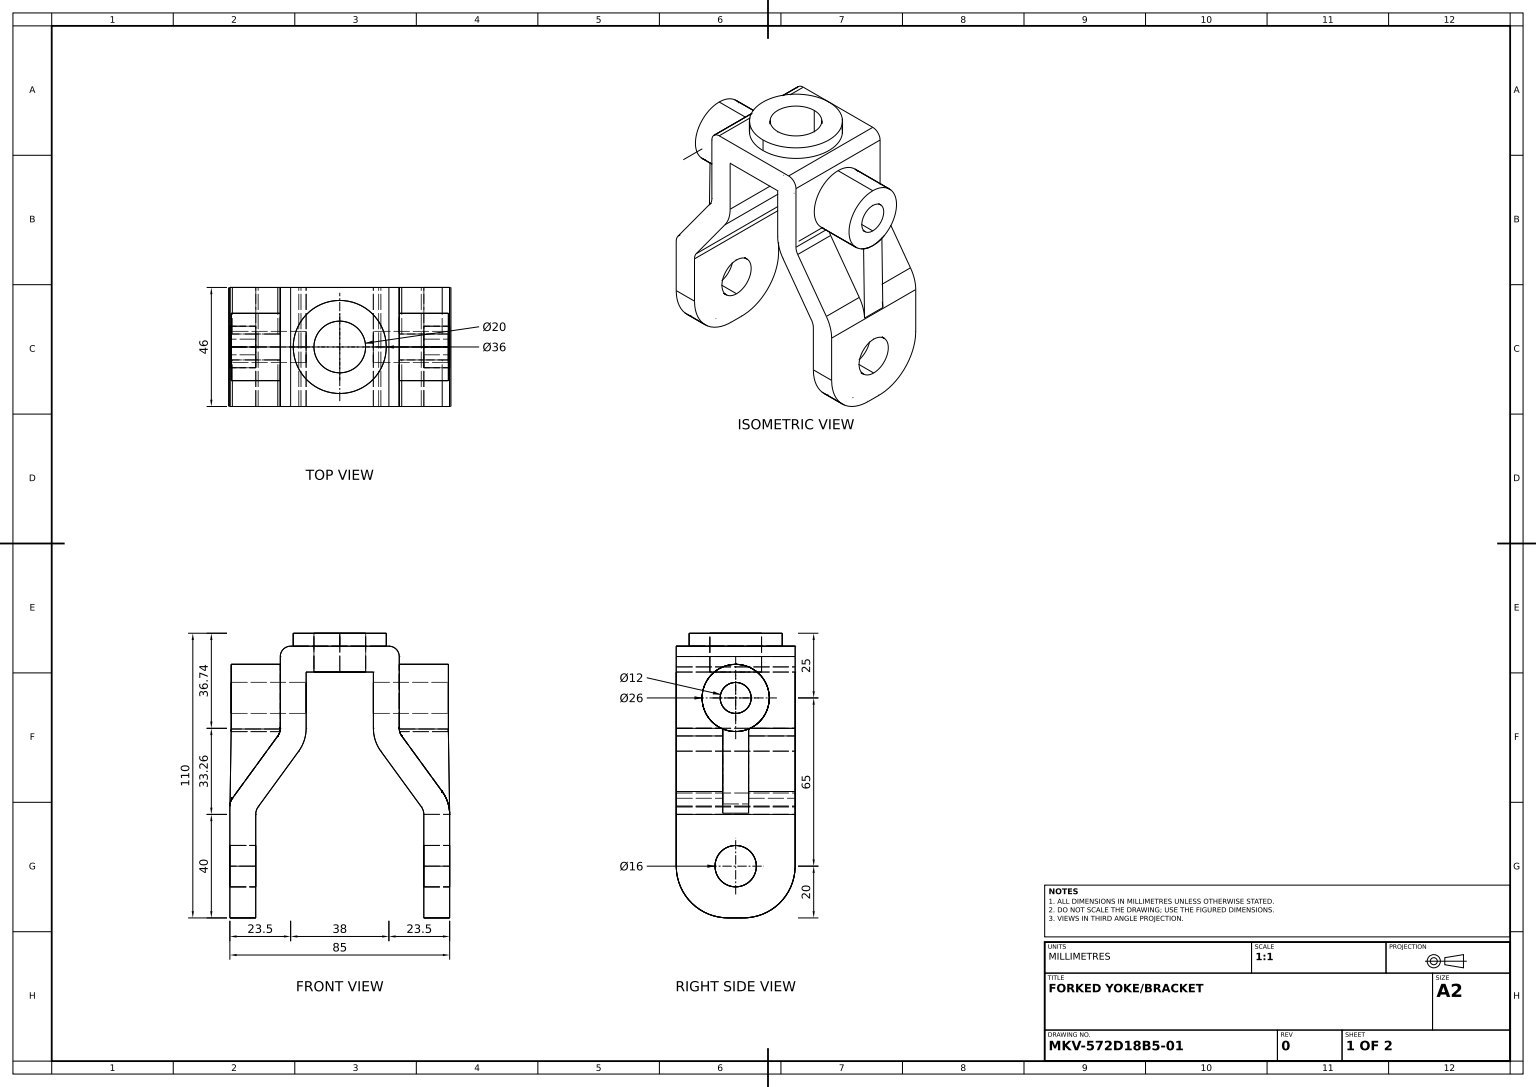
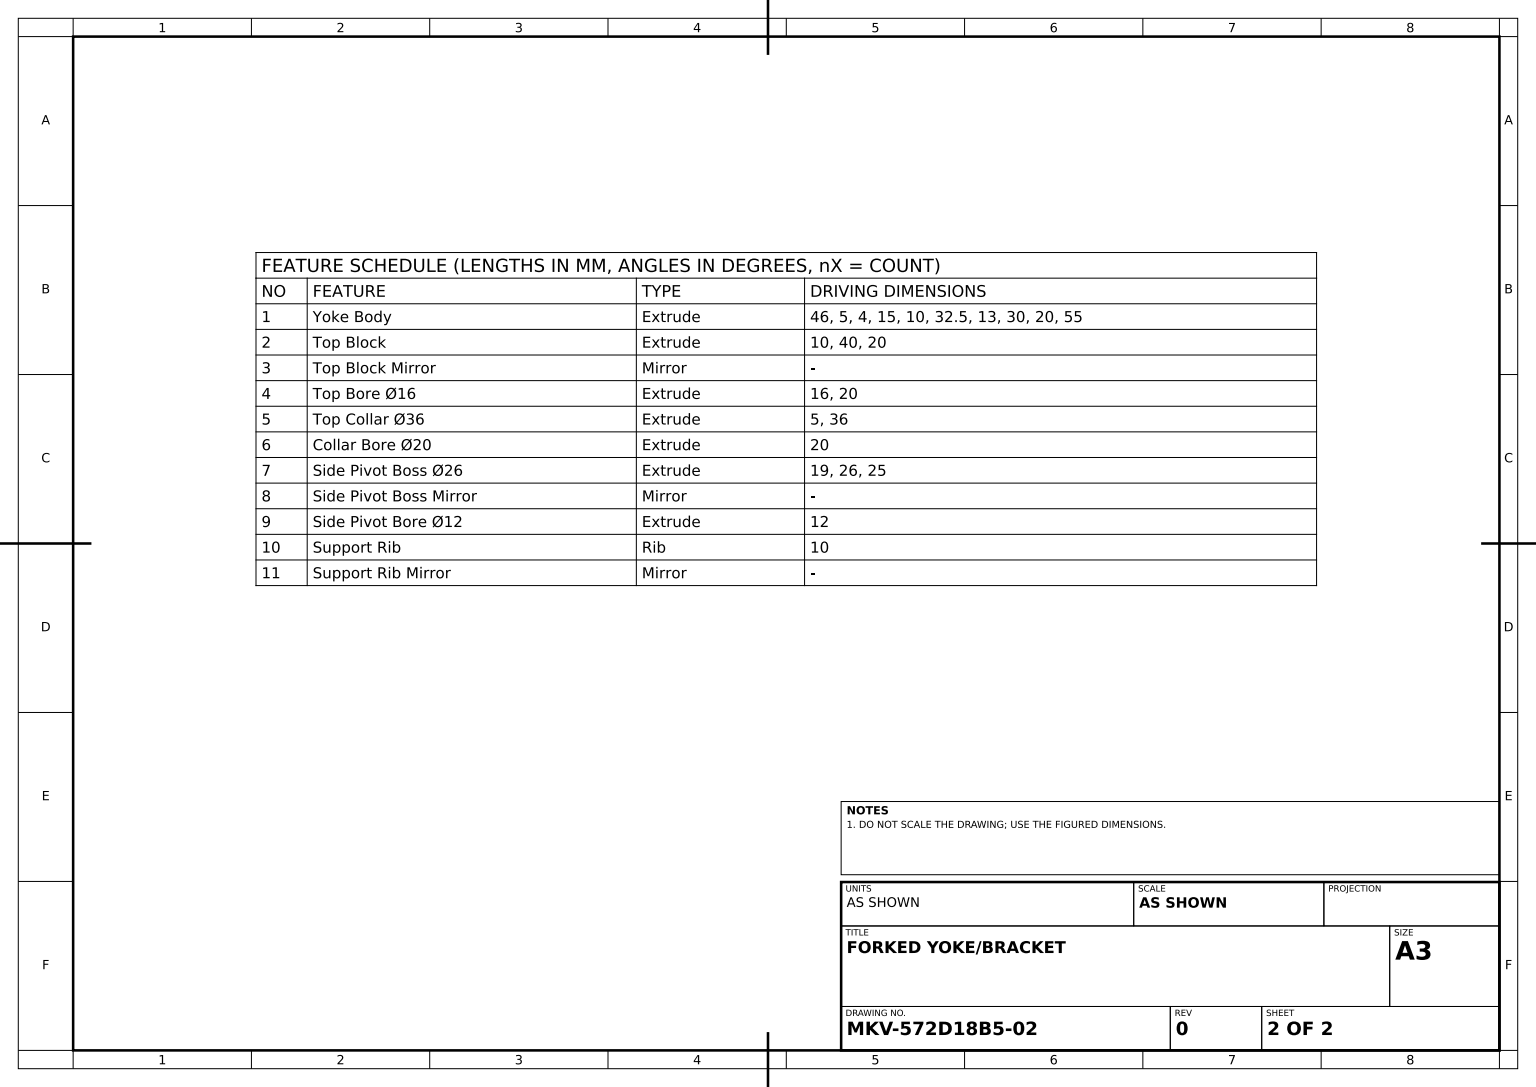
from build123d import *

# Parameters (mm, degrees)
YOKE_BODY_DEPTH           = 23
TOP_BLOCK_DEPTH           = 10
TOP_BORE_SKETCH_R         = 8
TOP_BORE_16_DEPTH         = 130.533779378
TOP_COLLAR_SKETCH_R       = 18
TOP_COLLAR_36_DEPTH       = 5
COLLAR_BORE_20_REACH      = 122.147
COLLAR_BORE_SKETCH_R      = 10
SIDE_PIVOT_BOSS_SKETCH_R  = 13
SIDE_PIVOT_BOSS_26_DEPTH  = 19
SIDE_PIVOT_BORE_SKETCH_R  = 6
SIDE_PIVOT_BORE_12_DEPTH  = 130.206230518
SUPPORT_RIB_REACH         = 108.584
SUPPORT_RIB_SKETCH_WALL_W = 247.172853136
SUPPORT_RIB_SKETCH_WALL_H = 10


with BuildPart() as part:
    # Yoke Profile Sketch → Yoke Body (new, symmetric)
    with BuildSketch(Plane.XY):
        with BuildLine():
            Line((19, 10), (-19, 10))
            ThreePointArc((-19, 10), (-21.828427125, 8.828427125), (-23, 6))
            Line((-23, 6), (-23, -21.741149913))
            ThreePointArc((-23, -21.741149913), (-23.246067912, -23.290385113), (-23.960051881, -24.687133484))
            Line((-23.960051881, -24.687133484), (-41.539948119, -48.795166343))
            ThreePointArc((-41.539948119, -48.795166343), (-42.253932088, -50.191914714), (-42.5, -51.741149913))
            Line((-42.5, -51.741149913), (-42.5, -71.741149913))
            Line((-42.5, -71.741149913), (-32.5, -71.741149913))
            Line((-32.5, -71.741149913), (-32.5, -55))
            ThreePointArc((-32.5, -55), (-32.253932088, -53.4507648), (-31.539948119, -52.054016429))
            Line((-31.539948119, -52.054016429), (-15.880155644, -30.579100626))
            ThreePointArc((-15.880155644, -30.579100626), (-13.738203736, -26.388855512), (-13, -21.741149913))
            Line((-13, -21.741149913), (-13, 0))
            Line((-13, 0), (13, 0))
            Line((13, 0), (13, -21.741149913))
            ThreePointArc((13, -21.741149913), (13.738203736, -26.388855512), (15.880155644, -30.579100626))
            Line((15.880155644, -30.579100626), (31.539948119, -52.054016429))
            ThreePointArc((31.539948119, -52.054016429), (32.253932088, -53.4507648), (32.5, -55))
            Line((32.5, -55), (32.5, -71.741149913))
            Line((32.5, -71.741149913), (42.5, -71.741149913))
            Line((42.5, -71.741149913), (42.5, -55))
            ThreePointArc((42.5, -55), (41.761796264, -50.352294401), (39.619844356, -46.162049287))
            Line((39.619844356, -46.162049287), (23.960051881, -24.687133484))
            ThreePointArc((23.960051881, -24.687133484), (23.246067912, -23.290385113), (23, -21.741149913))
            Line((23, -21.741149913), (23, 6))
            ThreePointArc((23, 6), (21.828427125, 8.828427125), (19, 10))
        make_face()
    extrude(amount=YOKE_BODY_DEPTH, both=True)

    # Top Block Sketch → Top Block (add)
    with BuildSketch(Plane(origin=(42.5, 0, 0), x_dir=(0, 0, -1), z_dir=(1, 0, 0))):
        with BuildLine():
            Line((-3, -95), (3, -95))
            ThreePointArc((3, -95), (17.142135624, -89.142135624), (23, -75))
            Line((23, -75), (23, -71.741149913))
            Line((23, -71.741149913), (-23, -71.741149913))
            Line((-23, -71.741149913), (-23, -75))
            ThreePointArc((-23, -75), (-17.142135624, -89.142135624), (-3, -95))
        make_face()
    top_block = extrude(amount=-TOP_BLOCK_DEPTH)

    # Top Block Mirror: Top Block across plane
    add(top_block.mirror(Plane(origin=(0, 0, 0), x_dir=(0, 0, 1), z_dir=(1, 0, 0))))

    # Top Bore Sketch → Top Bore Ø16 (cut, through all)
    with BuildSketch(Plane(origin=(42.5, 0, 0), x_dir=(0, 0, -1), z_dir=(1, 0, 0))):
        with Locations(Location((0, -75, 0), (0, 0, 90))):
            Circle(TOP_BORE_SKETCH_R)
    extrude(amount=-TOP_BORE_16_DEPTH, mode=Mode.SUBTRACT)

    # Top Collar Sketch → Top Collar Ø36 (add)
    with BuildSketch(Plane(origin=(0, 10, 0), x_dir=(1, 0, 0), z_dir=(0, 1, 0))):
        with Locations(Location((0, 0, 0), (0, 0, 90))):
            Circle(TOP_COLLAR_SKETCH_R)
    extrude(amount=TOP_COLLAR_36_DEPTH)

    # Collar Bore Sketch → Collar Bore Ø20 (cut, up to next)
    with BuildSketch(Plane(origin=(0, 15, 0), x_dir=(1, 0, 0), z_dir=(0, 1, 0)), mode=Mode.PRIVATE) as collar_bore_20_sk1:
        with Locations(Location((0, 0, 0), (0, 0, 270))):
            Circle(COLLAR_BORE_SKETCH_R)
    collar_bore_20_tool1 = extrude(collar_bore_20_sk1.sketch, amount=-COLLAR_BORE_20_REACH, mode=Mode.PRIVATE) & part.part
    add(collar_bore_20_tool1.solids().sort_by_distance((0, 15, 0))[0], mode=Mode.SUBTRACT)

    # Side Pivot Boss Sketch → Side Pivot Boss Ø26 (add)
    with BuildSketch(Plane(origin=(23, 0, 0), x_dir=(0, 0, -1), z_dir=(1, 0, 0))):
        with Locations(Location((0, -10, 0), (0, 0, 295.42268723))):
            Circle(SIDE_PIVOT_BOSS_SKETCH_R)
    side_pivot_boss_26 = extrude(amount=SIDE_PIVOT_BOSS_26_DEPTH)

    # Side Pivot Boss Mirror: Side Pivot Boss Ø26 across plane
    add(side_pivot_boss_26.mirror(Plane(origin=(0, 0, 0), x_dir=(0, 0, 1), z_dir=(1, 0, 0))))

    # Side Pivot Bore Sketch → Side Pivot Bore Ø12 (cut, through all)
    with BuildSketch(Plane(origin=(42, 0, 0), x_dir=(0, 0, -1), z_dir=(1, 0, 0))):
        with Locations(Location((0, -10, 0), (0, 0, 270))):
            Circle(SIDE_PIVOT_BORE_SKETCH_R)
    extrude(amount=-SIDE_PIVOT_BORE_12_DEPTH, mode=Mode.SUBTRACT)

    # Support Rib Sketch wall → Support Rib (add, up to next)
    with BuildSketch(Plane(origin=(42.25, -39, 0), x_dir=(0.015623093001, -0.999877952035, 0), z_dir=(0.999877952035, 0.015623093001, 0)), mode=Mode.PRIVATE) as support_rib_sk1:
        Rectangle(SUPPORT_RIB_SKETCH_WALL_W, SUPPORT_RIB_SKETCH_WALL_H)
    support_rib_tool1 = extrude(support_rib_sk1.sketch, amount=-SUPPORT_RIB_REACH, mode=Mode.PRIVATE) - part.part
    support_rib = support_rib_tool1.solids().sort_by_distance((42.25, -39, 0))[0]
    add(support_rib)

    # Support Rib Mirror: Support Rib across plane
    add(support_rib.mirror(Plane(origin=(0, 0, 0), x_dir=(0, 0, 1), z_dir=(1, 0, 0))))


solid = part.part
